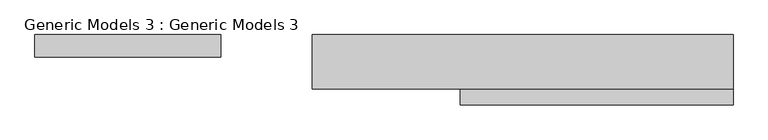
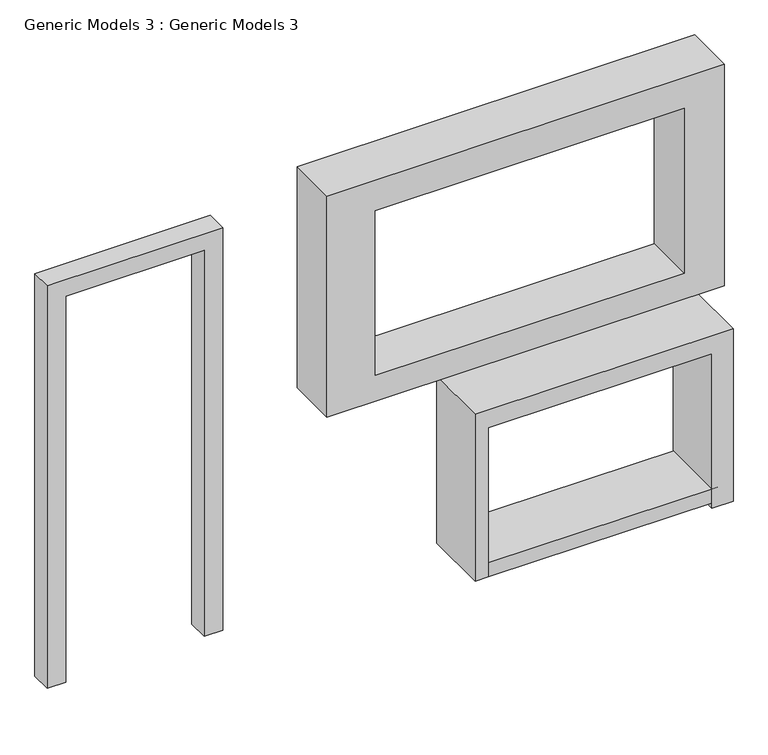
"""IFC4 building model written with IfcOpenShell, lengths in millimetres: proxy geometry, Generic Models 3 : Generic Models 3."""

from ifc_helpers import new_model, si_unit, frame, origin, origin_with_axes, place, context, project, spatial, polyline, outline, extrude, source, transform, mapped, element, save


def generic_models_3_generic_models_3_0a189295(model_context):
    return source(origin(), model_context, "Body", "SweptSolid", [
        extrude(outline(polyline([(0.0, -7084.2702714), (0.0, -6893.7702714), (2256.6794412, -6893.7702714), (2256.6794412, -3693.3702714), (-80.1205588, -3693.3702714), (-80.1205588, -3388.5702714), (2527.6003844, -3388.5702714), (2527.6003844, -7084.2702714), (0.0, -7084.2702714)])), frame((0.0, -12540.2383903, 0.0), z_axis=(0.0, 1.0, 0.0), x_axis=(0.0, 0.0, 1.0)), (0.0, 0.0, 1.0), 952.5),
        extrude(outline(polyline([(-3617.1702714, -11587.7383903), (-3617.1702714, -12540.2383903), (-6893.7702714, -12540.2383903), (-6893.7702714, -11587.7383903), (-3617.1702714, -11587.7383903)])), origin_with_axes(), (0.0, 0.0, 1.0), 210.6472196),
        extrude(outline(polyline([(6400.8, -3388.5702714), (6400.8, -9081.5517947), (3048.0, -9081.5517947), (3048.0, -3388.5702714), (6400.8, -3388.5702714)]), holes=[polyline([(5936.0869316, -3966.9367485), (3443.6107685, -3966.9367485), (3443.6107685, -8386.5367485), (5936.0869316, -8386.5367485), (5936.0869316, -3966.9367485)])]), frame((0.0, -12324.3383903, 0.0), z_axis=(0.0, 1.0, 0.0), x_axis=(0.0, 0.0, 1.0)), (0.0, 0.0, 1.0), 736.6),
        extrude(outline(polyline([(0.0, -12837.3702714), (0.0, -12570.6702714), (5845.1081495, -12570.6702714), (5845.1081495, -10589.4702714), (0.0, -10589.4702714), (0.0, -10322.7702714), (6096.0, -10322.7702714), (6096.0, -12837.3702714), (0.0, -12837.3702714)])), frame((0.0, -11892.5383903, 0.0), z_axis=(0.0, 1.0, 0.0), x_axis=(0.0, 0.0, 1.0)), (0.0, 0.0, 1.0), 304.8),
    ])


if __name__ == "__main__":
    model = new_model("IFC4")
    model_context = context("Model", 3, world=origin())
    ifc_project = project(units=[si_unit("LENGTHUNIT", "METRE", prefix="MILLI")], contexts=[model_context])
    site = spatial("IfcSite", under=ifc_project)
    building = spatial("IfcBuilding", under=site)
    placement = place(None, origin())
    generic_models_3_generic_models_3_shape = generic_models_3_generic_models_3_0a189295(model_context)
    element("IfcBuildingElementProxy", 1, Name="Generic Models 3 : Generic Models 3", ObjectType="Generic Models 3 : Generic Models 3", at=placement, inside=building, context=model_context, shape_type="MappedRepresentation", body=[
        mapped(generic_models_3_generic_models_3_shape, transform((0.0, 0.0, 0.0), x_axis=(1.0, 0.0, 0.0), y_axis=(0.0, 1.0, 0.0), z_axis=(0.0, 0.0, 1.0))),
    ])
    save(model, "model.ifc")
